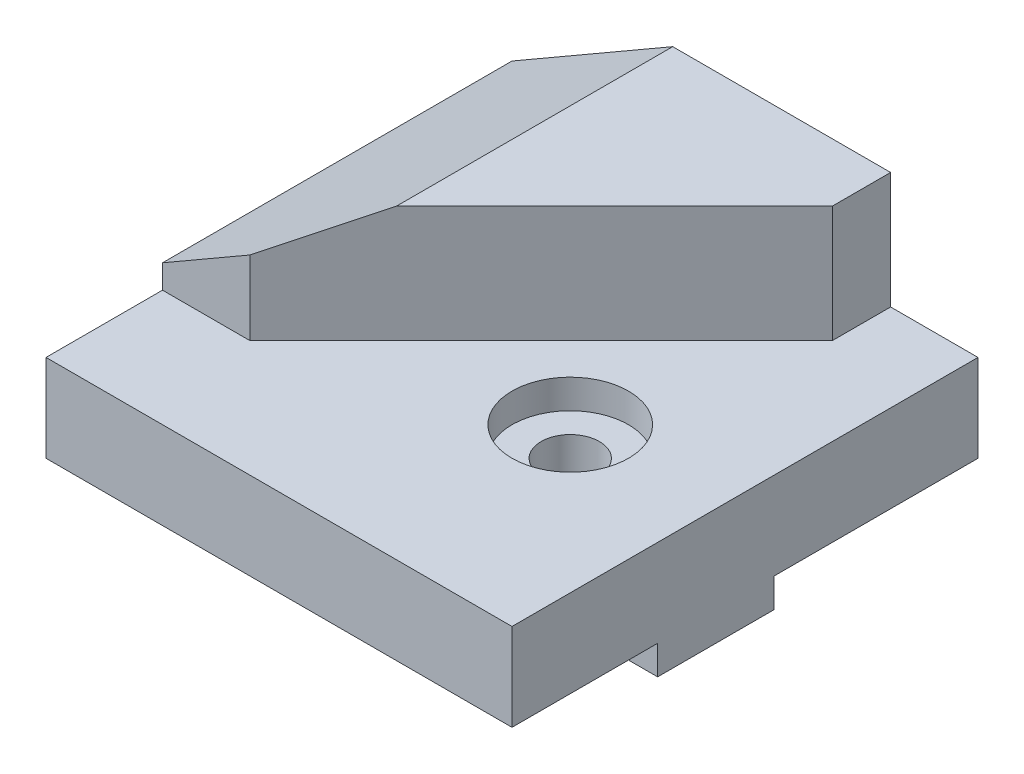
ISO-10303-21;
HEADER;
FILE_DESCRIPTION(('STEP AP214'),'2;1');
FILE_NAME('part.step','',(''),(''),'','','');
FILE_SCHEMA(('AUTOMOTIVE_DESIGN { 1 0 10303 214 1 1 1 1 }'));
ENDSEC;
DATA;
#1=APPLICATION_CONTEXT('core data for automotive mechanical design processes');
#2=APPLICATION_PROTOCOL_DEFINITION('international standard','automotive_design',2000,#1);
#3=PRODUCT_CONTEXT('',#1,'mechanical');
#4=PRODUCT('Part','Part','',(#3));
#5=PRODUCT_RELATED_PRODUCT_CATEGORY('part','',(#4));
#6=PRODUCT_DEFINITION_FORMATION('','',#4);
#7=PRODUCT_DEFINITION_CONTEXT('part definition',#1,'design');
#8=PRODUCT_DEFINITION('design','',#6,#7);
#9=PRODUCT_DEFINITION_SHAPE('','',#8);
#10=(LENGTH_UNIT() NAMED_UNIT(*) SI_UNIT(.MILLI.,.METRE.));
#11=(NAMED_UNIT(*) PLANE_ANGLE_UNIT() SI_UNIT($,.RADIAN.));
#12=(NAMED_UNIT(*) SI_UNIT($,.STERADIAN.) SOLID_ANGLE_UNIT());
#13=UNCERTAINTY_MEASURE_WITH_UNIT(LENGTH_MEASURE(1.E-05),#10,'distance_accuracy_value','');
#14=(GEOMETRIC_REPRESENTATION_CONTEXT(3) GLOBAL_UNCERTAINTY_ASSIGNED_CONTEXT((#13)) GLOBAL_UNIT_ASSIGNED_CONTEXT((#10,
#11,#12)) REPRESENTATION_CONTEXT('',''));
#15=CARTESIAN_POINT('',(0.,0.,0.));
#16=DIRECTION('',(0.,0.,1.));
#17=DIRECTION('',(1.,0.,0.));
#18=AXIS2_PLACEMENT_3D('',#15,#16,#17);
#19=CARTESIAN_POINT('',(0.,20.,0.));
#20=DIRECTION('',(0.,-1.,0.));
#21=DIRECTION('',(0.,0.,-1.));
#22=AXIS2_PLACEMENT_3D('',#19,#20,#21);
#23=PLANE('',#22);
#24=CARTESIAN_POINT('',(20.2398337208375,20.,-0.239833720837496));
#25=DIRECTION('',(0.,1.,0.));
#26=DIRECTION('',(0.,0.,1.));
#27=AXIS2_PLACEMENT_3D('',#24,#25,#26);
#28=CIRCLE('',#27,10.);
#29=CARTESIAN_POINT('',(20.2398337208375,20.,9.7601662791625));
#30=VERTEX_POINT('',#29);
#31=EDGE_CURVE('E510',#30,#30,#28,.T.);
#32=ORIENTED_EDGE('',*,*,#31,.F.);
#33=EDGE_LOOP('',(#32));
#34=FACE_BOUND('',#33,.T.);
#35=DIRECTION('',(1.,0.,0.));
#36=VECTOR('',#35,1.);
#37=CARTESIAN_POINT('',(45.2398337208375,20.,14.7601662791625));
#38=LINE('',#37,#36);
#39=CARTESIAN_POINT('',(-34.7601662791625,20.,14.7601662791625));
#40=VERTEX_POINT('',#39);
#41=CARTESIAN_POINT('',(-19.7601662791625,20.,14.7601662791625));
#42=VERTEX_POINT('',#41);
#43=EDGE_CURVE('E165',#40,#42,#38,.T.);
#44=ORIENTED_EDGE('',*,*,#43,.F.);
#45=DIRECTION('',(0.,0.,1.));
#46=VECTOR('',#45,1.);
#47=CARTESIAN_POINT('',(-34.7601662791625,20.,34.7601662791625));
#48=LINE('',#47,#46);
#49=CARTESIAN_POINT('',(-34.7601662791625,20.,34.7601662791625));
#50=VERTEX_POINT('',#49);
#51=EDGE_CURVE('E214',#40,#50,#48,.T.);
#52=ORIENTED_EDGE('',*,*,#51,.T.);
#53=DIRECTION('',(1.,0.,0.));
#54=VECTOR('',#53,1.);
#55=CARTESIAN_POINT('',(45.2398337208375,20.,34.7601662791625));
#56=LINE('',#55,#54);
#57=CARTESIAN_POINT('',(45.2398337208375,20.,34.7601662791625));
#58=VERTEX_POINT('',#57);
#59=EDGE_CURVE('E215',#50,#58,#56,.T.);
#60=ORIENTED_EDGE('',*,*,#59,.T.);
#61=DIRECTION('',(0.,0.,-1.));
#62=VECTOR('',#61,1.);
#63=CARTESIAN_POINT('',(45.2398337208375,20.,-45.2398337208375));
#64=LINE('',#63,#62);
#65=CARTESIAN_POINT('',(45.2398337208375,20.,-45.2398337208375));
#66=VERTEX_POINT('',#65);
#67=EDGE_CURVE('E218',#58,#66,#64,.T.);
#68=ORIENTED_EDGE('',*,*,#67,.T.);
#69=DIRECTION('',(-1.,0.,0.));
#70=VECTOR('',#69,1.);
#71=CARTESIAN_POINT('',(30.2398337208375,20.,-45.2398337208375));
#72=LINE('',#71,#70);
#73=CARTESIAN_POINT('',(30.2398337208375,20.,-45.2398337208375));
#74=VERTEX_POINT('',#73);
#75=EDGE_CURVE('E258',#66,#74,#72,.T.);
#76=ORIENTED_EDGE('',*,*,#75,.T.);
#77=DIRECTION('',(0.,0.,1.));
#78=VECTOR('',#77,1.);
#79=CARTESIAN_POINT('',(30.2398337208375,20.,-35.2398337208375));
#80=LINE('',#79,#78);
#81=CARTESIAN_POINT('',(30.2398337208375,20.,-35.2398337208375));
#82=VERTEX_POINT('',#81);
#83=EDGE_CURVE('E264',#74,#82,#80,.T.);
#84=ORIENTED_EDGE('',*,*,#83,.T.);
#85=DIRECTION('',(-0.707106781186547,0.,0.707106781186548));
#86=VECTOR('',#85,1.);
#87=CARTESIAN_POINT('',(30.2398337208375,20.,-35.2398337208375));
#88=LINE('',#87,#86);
#89=EDGE_CURVE('E274',#82,#42,#88,.T.);
#90=ORIENTED_EDGE('',*,*,#89,.T.);
#91=EDGE_LOOP('',(#44,#52,#60,#68,#76,#84,#90));
#92=FACE_BOUND('',#91,.T.);
#93=ADVANCED_FACE('F50',(#34,#92),#23,.F.);
#94=CARTESIAN_POINT('',(-34.7601662791625,20.,34.7601662791625));
#95=DIRECTION('',(1.,0.,0.));
#96=DIRECTION('',(0.,0.,-1.));
#97=AXIS2_PLACEMENT_3D('',#94,#95,#96);
#98=PLANE('',#97);
#99=DIRECTION('',(0.,-1.,0.));
#100=VECTOR('',#99,1.);
#101=CARTESIAN_POINT('',(-34.7601662791625,40.,14.7601662791625));
#102=LINE('',#101,#100);
#103=CARTESIAN_POINT('',(-34.7601662791625,24.0696274901458,14.7601662791625));
#104=VERTEX_POINT('',#103);
#105=EDGE_CURVE('E161',#104,#40,#102,.T.);
#106=ORIENTED_EDGE('',*,*,#105,.F.);
#107=DIRECTION('',(0.,0.,-1.));
#108=VECTOR('',#107,1.);
#109=CARTESIAN_POINT('',(-34.7601662791625,24.0696274901458,34.7611662791625));
#110=LINE('',#109,#108);
#111=CARTESIAN_POINT('',(-34.7601662791625,24.0696274901458,-45.2398337208375));
#112=VERTEX_POINT('',#111);
#113=EDGE_CURVE('E153',#104,#112,#110,.T.);
#114=ORIENTED_EDGE('',*,*,#113,.T.);
#115=DIRECTION('',(0.,-1.,0.));
#116=VECTOR('',#115,1.);
#117=CARTESIAN_POINT('',(-34.7601662791625,20.,-45.2398337208375));
#118=LINE('',#117,#116);
#119=CARTESIAN_POINT('',(-34.7601662791625,5.,-45.2398337208375));
#120=VERTEX_POINT('',#119);
#121=EDGE_CURVE('E160',#112,#120,#118,.T.);
#122=ORIENTED_EDGE('',*,*,#121,.T.);
#123=DIRECTION('',(0.,0.,1.));
#124=VECTOR('',#123,1.);
#125=CARTESIAN_POINT('',(-34.7601662791625,5.,-45.2398337208375));
#126=LINE('',#125,#124);
#127=CARTESIAN_POINT('',(-34.7601662791625,5.,-10.2398337208375));
#128=VERTEX_POINT('',#127);
#129=EDGE_CURVE('E205',#120,#128,#126,.T.);
#130=ORIENTED_EDGE('',*,*,#129,.T.);
#131=DIRECTION('',(0.,-1.,0.));
#132=VECTOR('',#131,1.);
#133=CARTESIAN_POINT('',(-34.7601662791625,5.,-10.2398337208375));
#134=LINE('',#133,#132);
#135=CARTESIAN_POINT('',(-34.7601662791625,0.,-10.2398337208375));
#136=VERTEX_POINT('',#135);
#137=EDGE_CURVE('E199',#128,#136,#134,.T.);
#138=ORIENTED_EDGE('',*,*,#137,.T.);
#139=DIRECTION('',(0.,0.,1.));
#140=VECTOR('',#139,1.);
#141=CARTESIAN_POINT('',(-34.7601662791625,0.,34.7601662791625));
#142=LINE('',#141,#140);
#143=CARTESIAN_POINT('',(-34.7601662791625,0.,9.76016627916252));
#144=VERTEX_POINT('',#143);
#145=EDGE_CURVE('E188',#136,#144,#142,.T.);
#146=ORIENTED_EDGE('',*,*,#145,.T.);
#147=DIRECTION('',(0.,1.,0.));
#148=VECTOR('',#147,1.);
#149=CARTESIAN_POINT('',(-34.7601662791625,0.,9.76016627916252));
#150=LINE('',#149,#148);
#151=CARTESIAN_POINT('',(-34.7601662791625,5.,9.76016627916252));
#152=VERTEX_POINT('',#151);
#153=EDGE_CURVE('E172',#144,#152,#150,.T.);
#154=ORIENTED_EDGE('',*,*,#153,.T.);
#155=DIRECTION('',(0.,0.,1.));
#156=VECTOR('',#155,1.);
#157=CARTESIAN_POINT('',(-34.7601662791625,5.,9.76016627916252));
#158=LINE('',#157,#156);
#159=CARTESIAN_POINT('',(-34.7601662791625,5.,34.7601662791625));
#160=VERTEX_POINT('',#159);
#161=EDGE_CURVE('E180',#152,#160,#158,.T.);
#162=ORIENTED_EDGE('',*,*,#161,.T.);
#163=DIRECTION('',(0.,-1.,0.));
#164=VECTOR('',#163,1.);
#165=CARTESIAN_POINT('',(-34.7601662791625,20.,34.7601662791625));
#166=LINE('',#165,#164);
#167=EDGE_CURVE('E11',#50,#160,#166,.T.);
#168=ORIENTED_EDGE('',*,*,#167,.F.);
#169=ORIENTED_EDGE('',*,*,#51,.F.);
#170=EDGE_LOOP('',(#106,#114,#122,#130,#138,#146,#154,#162,#168,#169));
#171=FACE_BOUND('',#170,.T.);
#172=ADVANCED_FACE('F47',(#171),#98,.F.);
#173=CARTESIAN_POINT('',(45.2398337208375,20.,34.7601662791625));
#174=DIRECTION('',(0.,0.,-1.));
#175=DIRECTION('',(-1.,0.,0.));
#176=AXIS2_PLACEMENT_3D('',#173,#174,#175);
#177=PLANE('',#176);
#178=ORIENTED_EDGE('',*,*,#167,.T.);
#179=DIRECTION('',(1.,0.,0.));
#180=VECTOR('',#179,1.);
#181=CARTESIAN_POINT('',(-34.7601662791625,5.,34.7601662791625));
#182=LINE('',#181,#180);
#183=CARTESIAN_POINT('',(45.2398337208375,5.,34.7601662791625));
#184=VERTEX_POINT('',#183);
#185=EDGE_CURVE('E190',#160,#184,#182,.T.);
#186=ORIENTED_EDGE('',*,*,#185,.T.);
#187=DIRECTION('',(0.,-1.,0.));
#188=VECTOR('',#187,1.);
#189=CARTESIAN_POINT('',(45.2398337208375,20.,34.7601662791625));
#190=LINE('',#189,#188);
#191=EDGE_CURVE('E54',#58,#184,#190,.T.);
#192=ORIENTED_EDGE('',*,*,#191,.F.);
#193=ORIENTED_EDGE('',*,*,#59,.F.);
#194=EDGE_LOOP('',(#178,#186,#192,#193));
#195=FACE_BOUND('',#194,.T.);
#196=ADVANCED_FACE('F234',(#195),#177,.F.);
#197=CARTESIAN_POINT('',(45.2398337208375,20.,-45.2398337208375));
#198=DIRECTION('',(-1.,0.,0.));
#199=DIRECTION('',(0.,0.,1.));
#200=AXIS2_PLACEMENT_3D('',#197,#198,#199);
#201=PLANE('',#200);
#202=DIRECTION('',(0.,-1.,0.));
#203=VECTOR('',#202,1.);
#204=CARTESIAN_POINT('',(45.2398337208375,20.,-45.2398337208375));
#205=LINE('',#204,#203);
#206=CARTESIAN_POINT('',(45.2398337208375,5.,-45.2398337208375));
#207=VERTEX_POINT('',#206);
#208=EDGE_CURVE('E222',#66,#207,#205,.T.);
#209=ORIENTED_EDGE('',*,*,#208,.F.);
#210=ORIENTED_EDGE('',*,*,#67,.F.);
#211=ORIENTED_EDGE('',*,*,#191,.T.);
#212=DIRECTION('',(0.,0.,1.));
#213=VECTOR('',#212,1.);
#214=CARTESIAN_POINT('',(45.2398337208375,5.,9.7601662791625));
#215=LINE('',#214,#213);
#216=CARTESIAN_POINT('',(45.2398337208375,5.,9.7601662791625));
#217=VERTEX_POINT('',#216);
#218=EDGE_CURVE('E178',#217,#184,#215,.T.);
#219=ORIENTED_EDGE('',*,*,#218,.F.);
#220=DIRECTION('',(0.,1.,0.));
#221=VECTOR('',#220,1.);
#222=CARTESIAN_POINT('',(45.2398337208375,0.,9.7601662791625));
#223=LINE('',#222,#221);
#224=CARTESIAN_POINT('',(45.2398337208375,0.,9.7601662791625));
#225=VERTEX_POINT('',#224);
#226=EDGE_CURVE('E185',#225,#217,#223,.T.);
#227=ORIENTED_EDGE('',*,*,#226,.F.);
#228=DIRECTION('',(0.,0.,-1.));
#229=VECTOR('',#228,1.);
#230=CARTESIAN_POINT('',(45.2398337208375,0.,-45.2398337208375));
#231=LINE('',#230,#229);
#232=CARTESIAN_POINT('',(45.2398337208375,0.,-10.2398337208375));
#233=VERTEX_POINT('',#232);
#234=EDGE_CURVE('E213',#225,#233,#231,.T.);
#235=ORIENTED_EDGE('',*,*,#234,.T.);
#236=DIRECTION('',(0.,-1.,0.));
#237=VECTOR('',#236,1.);
#238=CARTESIAN_POINT('',(45.2398337208375,5.,-10.2398337208375));
#239=LINE('',#238,#237);
#240=CARTESIAN_POINT('',(45.2398337208375,5.,-10.2398337208375));
#241=VERTEX_POINT('',#240);
#242=EDGE_CURVE('E204',#241,#233,#239,.T.);
#243=ORIENTED_EDGE('',*,*,#242,.F.);
#244=DIRECTION('',(0.,0.,1.));
#245=VECTOR('',#244,1.);
#246=CARTESIAN_POINT('',(45.2398337208375,5.,-45.2398337208375));
#247=LINE('',#246,#245);
#248=EDGE_CURVE('E184',#207,#241,#247,.T.);
#249=ORIENTED_EDGE('',*,*,#248,.F.);
#250=EDGE_LOOP('',(#209,#210,#211,#219,#227,#235,#243,#249));
#251=FACE_BOUND('',#250,.T.);
#252=ADVANCED_FACE('F229',(#251),#201,.F.);
#253=CARTESIAN_POINT('',(-34.7601662791625,20.,-45.2398337208375));
#254=DIRECTION('',(0.,0.,1.));
#255=DIRECTION('',(1.,0.,0.));
#256=AXIS2_PLACEMENT_3D('',#253,#254,#255);
#257=PLANE('',#256);
#258=ORIENTED_EDGE('',*,*,#121,.F.);
#259=DIRECTION('',(-0.866025403784442,-0.499999999999995,0.));
#260=VECTOR('',#259,1.);
#261=CARTESIAN_POINT('',(-7.1679517085961,40.,-45.2398337208375));
#262=LINE('',#261,#260);
#263=CARTESIAN_POINT('',(-7.1679517085961,40.,-45.2398337208375));
#264=VERTEX_POINT('',#263);
#265=EDGE_CURVE('E144',#264,#112,#262,.T.);
#266=ORIENTED_EDGE('',*,*,#265,.F.);
#267=DIRECTION('',(-1.,0.,0.));
#268=VECTOR('',#267,1.);
#269=CARTESIAN_POINT('',(-34.7601662791625,40.,-45.2398337208375));
#270=LINE('',#269,#268);
#271=CARTESIAN_POINT('',(30.2398337208375,40.,-45.2398337208375));
#272=VERTEX_POINT('',#271);
#273=EDGE_CURVE('E159',#272,#264,#270,.T.);
#274=ORIENTED_EDGE('',*,*,#273,.F.);
#275=DIRECTION('',(0.,1.,0.));
#276=VECTOR('',#275,1.);
#277=CARTESIAN_POINT('',(30.2398337208375,20.,-45.2398337208375));
#278=LINE('',#277,#276);
#279=EDGE_CURVE('E66',#74,#272,#278,.T.);
#280=ORIENTED_EDGE('',*,*,#279,.F.);
#281=ORIENTED_EDGE('',*,*,#75,.F.);
#282=ORIENTED_EDGE('',*,*,#208,.T.);
#283=DIRECTION('',(1.,0.,0.));
#284=VECTOR('',#283,1.);
#285=CARTESIAN_POINT('',(-34.7601662791625,5.,-45.2398337208375));
#286=LINE('',#285,#284);
#287=EDGE_CURVE('E193',#120,#207,#286,.T.);
#288=ORIENTED_EDGE('',*,*,#287,.F.);
#289=EDGE_LOOP('',(#258,#266,#274,#280,#281,#282,#288));
#290=FACE_BOUND('',#289,.T.);
#291=ADVANCED_FACE('F158',(#290),#257,.F.);
#292=CARTESIAN_POINT('',(0.,0.,0.));
#293=DIRECTION('',(0.,-1.,0.));
#294=DIRECTION('',(0.,0.,-1.));
#295=AXIS2_PLACEMENT_3D('',#292,#293,#294);
#296=PLANE('',#295);
#297=DIRECTION('',(1.,0.,0.));
#298=VECTOR('',#297,1.);
#299=CARTESIAN_POINT('',(-34.7601662791625,0.,9.76016627916252));
#300=LINE('',#299,#298);
#301=EDGE_CURVE('E181',#144,#225,#300,.T.);
#302=ORIENTED_EDGE('',*,*,#301,.F.);
#303=ORIENTED_EDGE('',*,*,#145,.F.);
#304=DIRECTION('',(1.,0.,0.));
#305=VECTOR('',#304,1.);
#306=CARTESIAN_POINT('',(-34.7601662791625,0.,-10.2398337208375));
#307=LINE('',#306,#305);
#308=EDGE_CURVE('E168',#136,#233,#307,.T.);
#309=ORIENTED_EDGE('',*,*,#308,.T.);
#310=ORIENTED_EDGE('',*,*,#234,.F.);
#311=EDGE_LOOP('',(#302,#303,#309,#310));
#312=FACE_BOUND('',#311,.T.);
#313=ADVANCED_FACE('F247',(#312),#296,.T.);
#314=CARTESIAN_POINT('',(-34.7601662791625,5.,-10.2398337208375));
#315=DIRECTION('',(0.,0.,1.));
#316=DIRECTION('',(0.,-1.,0.));
#317=AXIS2_PLACEMENT_3D('',#314,#315,#316);
#318=PLANE('',#317);
#319=ORIENTED_EDGE('',*,*,#242,.T.);
#320=ORIENTED_EDGE('',*,*,#308,.F.);
#321=ORIENTED_EDGE('',*,*,#137,.F.);
#322=DIRECTION('',(1.,0.,0.));
#323=VECTOR('',#322,1.);
#324=CARTESIAN_POINT('',(-34.7601662791625,5.,-10.2398337208375));
#325=LINE('',#324,#323);
#326=EDGE_CURVE('E197',#128,#241,#325,.T.);
#327=ORIENTED_EDGE('',*,*,#326,.T.);
#328=EDGE_LOOP('',(#319,#320,#321,#327));
#329=FACE_BOUND('',#328,.T.);
#330=ADVANCED_FACE('F255',(#329),#318,.F.);
#331=CARTESIAN_POINT('',(-34.7601662791625,5.,-45.2398337208375));
#332=DIRECTION('',(0.,1.,0.));
#333=DIRECTION('',(0.,0.,1.));
#334=AXIS2_PLACEMENT_3D('',#331,#332,#333);
#335=PLANE('',#334);
#336=ORIENTED_EDGE('',*,*,#248,.T.);
#337=ORIENTED_EDGE('',*,*,#326,.F.);
#338=ORIENTED_EDGE('',*,*,#129,.F.);
#339=ORIENTED_EDGE('',*,*,#287,.T.);
#340=EDGE_LOOP('',(#336,#337,#338,#339));
#341=FACE_BOUND('',#340,.T.);
#342=ADVANCED_FACE('F259',(#341),#335,.F.);
#343=CARTESIAN_POINT('',(-34.7601662791625,5.,9.76016627916252));
#344=DIRECTION('',(0.,1.,0.));
#345=DIRECTION('',(0.,0.,1.));
#346=AXIS2_PLACEMENT_3D('',#343,#344,#345);
#347=PLANE('',#346);
#348=ORIENTED_EDGE('',*,*,#218,.T.);
#349=ORIENTED_EDGE('',*,*,#185,.F.);
#350=ORIENTED_EDGE('',*,*,#161,.F.);
#351=DIRECTION('',(1.,0.,0.));
#352=VECTOR('',#351,1.);
#353=CARTESIAN_POINT('',(-34.7601662791625,5.,9.76016627916252));
#354=LINE('',#353,#352);
#355=EDGE_CURVE('E194',#152,#217,#354,.T.);
#356=ORIENTED_EDGE('',*,*,#355,.T.);
#357=EDGE_LOOP('',(#348,#349,#350,#356));
#358=FACE_BOUND('',#357,.T.);
#359=ADVANCED_FACE('F238',(#358),#347,.F.);
#360=CARTESIAN_POINT('',(-34.7601662791625,0.,9.76016627916252));
#361=DIRECTION('',(0.,0.,-1.));
#362=DIRECTION('',(-1.,0.,0.));
#363=AXIS2_PLACEMENT_3D('',#360,#361,#362);
#364=PLANE('',#363);
#365=ORIENTED_EDGE('',*,*,#226,.T.);
#366=ORIENTED_EDGE('',*,*,#355,.F.);
#367=ORIENTED_EDGE('',*,*,#153,.F.);
#368=ORIENTED_EDGE('',*,*,#301,.T.);
#369=EDGE_LOOP('',(#365,#366,#367,#368));
#370=FACE_BOUND('',#369,.T.);
#371=ADVANCED_FACE('F244',(#370),#364,.F.);
#372=CARTESIAN_POINT('',(45.2398337208375,40.,14.7601662791625));
#373=DIRECTION('',(0.,0.,-1.));
#374=DIRECTION('',(-1.,0.,0.));
#375=AXIS2_PLACEMENT_3D('',#372,#373,#374);
#376=PLANE('',#375);
#377=DIRECTION('',(0.,1.,0.));
#378=VECTOR('',#377,1.);
#379=CARTESIAN_POINT('',(-19.7601662791625,20.,14.7601662791625));
#380=LINE('',#379,#378);
#381=CARTESIAN_POINT('',(-19.7601662791625,32.7298815279901,14.7601662791625));
#382=VERTEX_POINT('',#381);
#383=EDGE_CURVE('E261',#42,#382,#380,.T.);
#384=ORIENTED_EDGE('',*,*,#383,.T.);
#385=DIRECTION('',(0.866025403784442,0.499999999999995,0.));
#386=VECTOR('',#385,1.);
#387=CARTESIAN_POINT('',(-7.16795170859611,40.,14.7601662791625));
#388=LINE('',#387,#386);
#389=EDGE_CURVE('E61',#104,#382,#388,.T.);
#390=ORIENTED_EDGE('',*,*,#389,.F.);
#391=ORIENTED_EDGE('',*,*,#105,.T.);
#392=ORIENTED_EDGE('',*,*,#43,.T.);
#393=EDGE_LOOP('',(#384,#390,#391,#392));
#394=FACE_BOUND('',#393,.T.);
#395=ADVANCED_FACE('F282',(#394),#376,.F.);
#396=CARTESIAN_POINT('',(0.,40.,0.));
#397=DIRECTION('',(0.,-1.,0.));
#398=DIRECTION('',(0.,0.,-1.));
#399=AXIS2_PLACEMENT_3D('',#396,#397,#398);
#400=PLANE('',#399);
#401=ORIENTED_EDGE('',*,*,#273,.T.);
#402=DIRECTION('',(0.,0.,-1.));
#403=VECTOR('',#402,1.);
#404=CARTESIAN_POINT('',(-7.1679517085961,40.,34.7611662791625));
#405=LINE('',#404,#403);
#406=CARTESIAN_POINT('',(-7.1679517085961,40.,2.16795170859614));
#407=VERTEX_POINT('',#406);
#408=EDGE_CURVE('E142',#407,#264,#405,.T.);
#409=ORIENTED_EDGE('',*,*,#408,.F.);
#410=DIRECTION('',(-0.707106781186547,0.,0.707106781186548));
#411=VECTOR('',#410,1.);
#412=CARTESIAN_POINT('',(30.2398337208375,40.,-35.2398337208375));
#413=LINE('',#412,#411);
#414=CARTESIAN_POINT('',(30.2398337208375,40.,-35.2398337208375));
#415=VERTEX_POINT('',#414);
#416=EDGE_CURVE('E275',#415,#407,#413,.T.);
#417=ORIENTED_EDGE('',*,*,#416,.F.);
#418=DIRECTION('',(0.,0.,1.));
#419=VECTOR('',#418,1.);
#420=CARTESIAN_POINT('',(30.2398337208375,40.,-35.2398337208375));
#421=LINE('',#420,#419);
#422=EDGE_CURVE('E162',#272,#415,#421,.T.);
#423=ORIENTED_EDGE('',*,*,#422,.F.);
#424=EDGE_LOOP('',(#401,#409,#417,#423));
#425=FACE_BOUND('',#424,.T.);
#426=ADVANCED_FACE('F163',(#425),#400,.F.);
#427=CARTESIAN_POINT('',(30.2398337208375,20.,-35.2398337208375));
#428=DIRECTION('',(-1.,0.,0.));
#429=DIRECTION('',(0.,0.,1.));
#430=AXIS2_PLACEMENT_3D('',#427,#428,#429);
#431=PLANE('',#430);
#432=ORIENTED_EDGE('',*,*,#422,.T.);
#433=DIRECTION('',(0.,1.,0.));
#434=VECTOR('',#433,1.);
#435=CARTESIAN_POINT('',(30.2398337208375,20.,-35.2398337208375));
#436=LINE('',#435,#434);
#437=EDGE_CURVE('E169',#82,#415,#436,.T.);
#438=ORIENTED_EDGE('',*,*,#437,.F.);
#439=ORIENTED_EDGE('',*,*,#83,.F.);
#440=ORIENTED_EDGE('',*,*,#279,.T.);
#441=EDGE_LOOP('',(#432,#438,#439,#440));
#442=FACE_BOUND('',#441,.T.);
#443=ADVANCED_FACE('F273',(#442),#431,.F.);
#444=CARTESIAN_POINT('',(30.2398337208375,20.,-35.2398337208375));
#445=DIRECTION('',(-0.707106781186548,0.,-0.707106781186547));
#446=DIRECTION('',(-0.707106781186547,0.,0.707106781186548));
#447=AXIS2_PLACEMENT_3D('',#444,#445,#446);
#448=PLANE('',#447);
#449=ORIENTED_EDGE('',*,*,#416,.T.);
#450=DIRECTION('',(0.654653670707978,0.377964473009222,-0.654653670707979));
#451=VECTOR('',#450,1.);
#452=CARTESIAN_POINT('',(-21.1364722388389,31.9352709116836,16.1364722388389));
#453=LINE('',#452,#451);
#454=EDGE_CURVE('E149',#382,#407,#453,.T.);
#455=ORIENTED_EDGE('',*,*,#454,.F.);
#456=ORIENTED_EDGE('',*,*,#383,.F.);
#457=ORIENTED_EDGE('',*,*,#89,.F.);
#458=ORIENTED_EDGE('',*,*,#437,.T.);
#459=EDGE_LOOP('',(#449,#455,#456,#457,#458));
#460=FACE_BOUND('',#459,.T.);
#461=ADVANCED_FACE('F272',(#460),#448,.F.);
#462=CARTESIAN_POINT('',(-7.1679517085961,40.,34.7611662791625));
#463=DIRECTION('',(0.499999999999995,-0.866025403784442,0.));
#464=DIRECTION('',(0.866025403784442,0.499999999999995,0.));
#465=AXIS2_PLACEMENT_3D('',#462,#463,#464);
#466=PLANE('',#465);
#467=ORIENTED_EDGE('',*,*,#389,.T.);
#468=ORIENTED_EDGE('',*,*,#454,.T.);
#469=ORIENTED_EDGE('',*,*,#408,.T.);
#470=ORIENTED_EDGE('',*,*,#265,.T.);
#471=ORIENTED_EDGE('',*,*,#113,.F.);
#472=EDGE_LOOP('',(#467,#468,#469,#470,#471));
#473=FACE_BOUND('',#472,.T.);
#474=ADVANCED_FACE('F141',(#473),#466,.F.);
#475=CARTESIAN_POINT('',(20.2398337208375,15.,-0.239833720837496));
#476=DIRECTION('',(0.,1.,0.));
#477=DIRECTION('',(0.,0.,1.));
#478=AXIS2_PLACEMENT_3D('',#475,#476,#477);
#479=CYLINDRICAL_SURFACE('',#478,10.);
#480=CARTESIAN_POINT('',(20.2398337208375,15.,-0.239833720837496));
#481=DIRECTION('',(0.,1.,0.));
#482=DIRECTION('',(0.,0.,1.));
#483=AXIS2_PLACEMENT_3D('',#480,#481,#482);
#484=CIRCLE('',#483,10.);
#485=CARTESIAN_POINT('',(20.2398337208375,15.,9.7601662791625));
#486=VERTEX_POINT('',#485);
#487=EDGE_CURVE('E512',#486,#486,#484,.T.);
#488=ORIENTED_EDGE('',*,*,#487,.F.);
#489=EDGE_LOOP('',(#488));
#490=FACE_BOUND('',#489,.T.);
#491=ORIENTED_EDGE('',*,*,#31,.T.);
#492=EDGE_LOOP('',(#491));
#493=FACE_BOUND('',#492,.T.);
#494=ADVANCED_FACE('F382',(#490,#493),#479,.F.);
#495=CARTESIAN_POINT('',(20.2398337208375,15.,-0.239833720837496));
#496=DIRECTION('',(0.,1.,0.));
#497=DIRECTION('',(0.,0.,1.));
#498=AXIS2_PLACEMENT_3D('',#495,#496,#497);
#499=PLANE('',#498);
#500=CARTESIAN_POINT('',(20.2398337208375,15.,-0.239833720837496));
#501=DIRECTION('',(0.,1.,0.));
#502=DIRECTION('',(0.,0.,1.));
#503=AXIS2_PLACEMENT_3D('',#500,#501,#502);
#504=CIRCLE('',#503,5.);
#505=CARTESIAN_POINT('',(20.2398337208375,15.,4.7601662791625));
#506=VERTEX_POINT('',#505);
#507=EDGE_CURVE('E507',#506,#506,#504,.T.);
#508=ORIENTED_EDGE('',*,*,#507,.F.);
#509=EDGE_LOOP('',(#508));
#510=FACE_BOUND('',#509,.T.);
#511=ORIENTED_EDGE('',*,*,#487,.T.);
#512=EDGE_LOOP('',(#511));
#513=FACE_BOUND('',#512,.T.);
#514=ADVANCED_FACE('F391',(#510,#513),#499,.T.);
#515=CARTESIAN_POINT('',(20.2398337208375,5.,-0.239833720837496));
#516=DIRECTION('',(0.,1.,0.));
#517=DIRECTION('',(0.,0.,1.));
#518=AXIS2_PLACEMENT_3D('',#515,#516,#517);
#519=CYLINDRICAL_SURFACE('',#518,5.);
#520=CARTESIAN_POINT('',(20.2398337208375,5.,-0.239833720837496));
#521=DIRECTION('',(0.,1.,0.));
#522=DIRECTION('',(0.,0.,1.));
#523=AXIS2_PLACEMENT_3D('',#520,#521,#522);
#524=CIRCLE('',#523,5.);
#525=CARTESIAN_POINT('',(20.2398337208375,5.,4.7601662791625));
#526=VERTEX_POINT('',#525);
#527=EDGE_CURVE('E506',#526,#526,#524,.T.);
#528=ORIENTED_EDGE('',*,*,#527,.F.);
#529=EDGE_LOOP('',(#528));
#530=FACE_BOUND('',#529,.T.);
#531=ORIENTED_EDGE('',*,*,#507,.T.);
#532=EDGE_LOOP('',(#531));
#533=FACE_BOUND('',#532,.T.);
#534=ADVANCED_FACE('F404',(#530,#533),#519,.F.);
#535=CARTESIAN_POINT('',(20.2398337208375,5.,-0.239833720837496));
#536=DIRECTION('',(0.,1.,0.));
#537=DIRECTION('',(0.,0.,1.));
#538=AXIS2_PLACEMENT_3D('',#535,#536,#537);
#539=PLANE('',#538);
#540=ORIENTED_EDGE('',*,*,#527,.T.);
#541=EDGE_LOOP('',(#540));
#542=FACE_BOUND('',#541,.T.);
#543=ADVANCED_FACE('F412',(#542),#539,.T.);
#544=CLOSED_SHELL('',(#93,#172,#196,#252,#291,#313,#330,#342,#359,#371,#395,#426,#443,#461,#474,
#494,#514,#534,#543));
#545=MANIFOLD_SOLID_BREP('B2',#544);
#546=ADVANCED_BREP_SHAPE_REPRESENTATION('',(#18,#545),#14);
#547=SHAPE_DEFINITION_REPRESENTATION(#9,#546);
ENDSEC;
END-ISO-10303-21;
